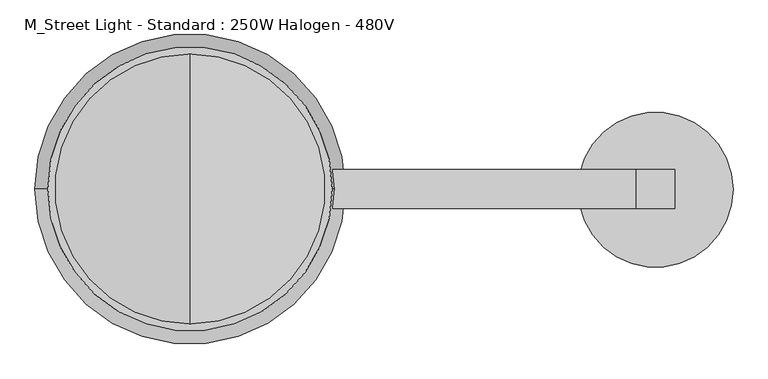
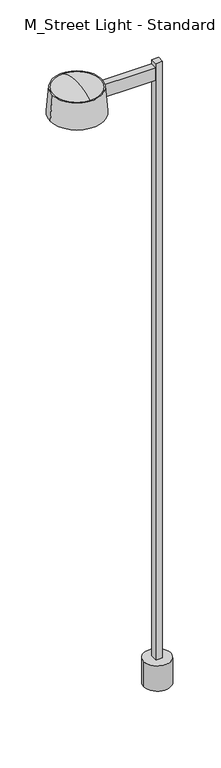
"""IFC4 building model written with IfcOpenShell, lengths in millimetres: light fixture geometry, M_Street Light - Standard : 250W Halogen - 480V."""

from ifc_helpers import new_model, si_unit, point, frame, origin, origin_with_axes, origin_2d, place, context, project, spatial, polyline, circle_curve, ellipse_curve, trimmed, segment, composite_curve, outline, extrude, source, transform, mapped, element, save
from ifc_brep_helpers import plane_surface, revolved_surface, advanced_brep


def m_street_light_standard_250w_halogen_480v_204dbcbb(model_context):
    return source(origin(), model_context, "Body", "SolidModel", [
        extrude(outline(composite_curve([segment(trimmed(circle_curve(origin_2d(), 152.4), [point((-152.4, 0.0))], [point((152.4, 0.0))], False, "CARTESIAN"), True, "CONTINUOUS"), segment(trimmed(circle_curve(origin_2d(), 152.4), [point((152.4, 0.0))], [point((-152.4, 0.0))], False, "CARTESIAN"), True, "CONTINUOUS")], self_intersect=False)), origin_with_axes(), (0.0, 0.0, 1.0), 304.8),
        extrude(outline(polyline([(38.1, 38.1), (38.1, -38.1), (-38.1, -38.1), (-38.1, 38.1), (38.1, 38.1)])), frame((0.0, 0.0, 304.8), z_axis=(0.0, 0.0, 1.0), x_axis=(1.0, 0.0, 0.0)), (0.0, 0.0, 1.0), 7195.2),
        extrude(outline(polyline([(-914.4, 38.1), (-38.1, 38.1), (-38.1, -38.1), (-914.4, -38.1), (-914.4, 38.1)])), frame((0.0, 0.0, 7296.8), z_axis=(0.0, 0.0, 1.0), x_axis=(1.0, 0.0, 0.0)), (0.0, 0.0, 1.0), 152.4),
        advanced_brep(
        [(-1193.8, 0.0, 7500.0), (-635.0, 0.0, 7500.0), (-1219.2, 0.0, 7195.2), (-609.6, 0.0, 7195.2)],
        [
            (0, 1, circle_curve(frame((-914.4, 0.0, 7500.0), z_axis=(0.0, 0.0, 1.0), x_axis=(-1.0, 0.0, 0.0)), 279.4)),
            (1, 0, circle_curve(frame((-914.4, 0.0, 7500.0), z_axis=(0.0, 0.0, 1.0), x_axis=(1.0, 0.0, 0.0)), 279.4)),
            (2, 3, circle_curve(frame((-914.4, 0.0, 7195.2), z_axis=(0.0, 0.0, -1.0), x_axis=(1.0, 0.0, 0.0)), 304.8)),
            (3, 2, circle_curve(frame((-914.4, 0.0, 7195.2), z_axis=(0.0, 0.0, -1.0), x_axis=(-1.0, 0.0, 0.0)), 304.8)),
            (3, 1),
            (0, 2),
        ],
        [
            plane_surface(frame((-914.4, 0.0, 7500.0), z_axis=(0.0, 0.0, 1.0), x_axis=(0.0, -1.0, 0.0))),
            plane_surface(frame((-914.4, 0.0, 7195.2), z_axis=(0.0, 0.0, -1.0), x_axis=(0.0, -1.0, 0.0))),
            revolved_surface(polyline([(-1193.8, 0.0, 7500.0), (-1219.2, 0.0, 7195.2)]), (-914.4, 0.0, 10852.8), (0.0, 0.0, -1.0)),
            revolved_surface(polyline([(-635.0, 0.0, 7500.0), (-609.6, 0.0, 7195.2)]), (-914.4, 0.0, 10852.8), (0.0, 0.0, -1.0)),
        ],
        [
            (0, [[1, 2]]),
            (1, [[3, 4]]),
            (2, [[-4, 5, -1, 6]]),
            (3, [[-3, -6, -2, -5]]),
        ],
    ),
        advanced_brep(
        [(-914.4, -266.7, 7500.0), (-914.4, 266.7, 7500.0), (-914.4, 0.0, 7571.4620496), (-914.4, -228.6332063, 7500.0), (-914.4, 228.6332063, 7500.0), (-914.4, 0.0, 7558.7620496)],
        [
            (0, 1, circle_curve(frame((-914.4, 0.0, 7500.0), z_axis=(0.0, 0.0, 1.0), x_axis=(0.0, 1.0, 0.0)), 266.7)),
            (1, 2, circle_curve(frame((-914.4, -28.9924067, 6929.8609147), z_axis=(1.0, 0.0, 0.0), x_axis=(0.0, 0.0, 1.0)), 642.2558493)),
            (2, 0, circle_curve(frame((-914.4, 28.9924067, 6929.8609147), z_axis=(1.0, 0.0, 0.0), x_axis=(0.0, 0.0, 1.0)), 642.2558493)),
            (1, 0, circle_curve(frame((-914.4, 0.0, 7500.0), z_axis=(0.0, 0.0, 1.0), x_axis=(0.0, 1.0, 0.0)), 266.7)),
            (3, 4, circle_curve(frame((-914.4, 0.0, 7500.0), z_axis=(0.0, 0.0, 1.0), x_axis=(0.0, 1.0, 0.0)), 228.6332063)),
            (4, 1),
            (0, 3),
            (4, 3, circle_curve(frame((-914.4, 0.0, 7500.0), z_axis=(0.0, 0.0, 1.0), x_axis=(0.0, 1.0, 0.0)), 228.6332063)),
            (5, 4),
            (3, 5),
        ],
        [
            revolved_surface(trimmed(ellipse_curve(frame((-914.4, -28.9924067, 6929.8609147), z_axis=(-1.0, 0.0, 0.0), x_axis=(0.0, 0.0, 1.0)), 642.2558493, 642.2558493), [point((-914.4, 0.0, 7571.4620496))], [point((-914.4, 266.7, 7500.0))], True, "CARTESIAN"), (-914.4, 0.0, 7423.8), (0.0, 0.0, -1.0)),
            plane_surface(frame((-914.4, 0.0, 7500.0), z_axis=(0.0, 0.0, -1.0), x_axis=(0.0, 1.0, 0.0))),
            revolved_surface(polyline([(-914.4, 228.6332063, 7500.0), (-914.4, 0.0, 7558.7620496)]), (-914.4, 0.0, 7423.8), (0.0, 0.0, -1.0)),
        ],
        [
            (0, [[1, 2, 3]]),
            (0, [[4, -3, -2]]),
            (1, [[5, 6, -1, 7]]),
            (1, [[8, -7, -4, -6]]),
            (2, [[9, -5, 10]]),
            (2, [[-10, -8, -9]]),
        ],
    ),
        advanced_brep(
        [(-914.4, -228.6332063, 7195.2), (-914.4, 228.6332063, 7195.2), (-914.4, 0.0, 7136.4379504), (-914.4, -266.7, 7195.2), (-914.4, 266.7, 7195.2), (-914.4, 0.0, 7123.7379504)],
        [
            (0, 1, circle_curve(frame((-914.4, 0.0, 7195.2), z_axis=(0.0, 0.0, 1.0), x_axis=(0.0, 1.0, 0.0)), 228.6332063)),
            (1, 2),
            (2, 0),
            (1, 0, circle_curve(frame((-914.4, 0.0, 7195.2), z_axis=(0.0, 0.0, 1.0), x_axis=(0.0, 1.0, 0.0)), 228.6332063)),
            (3, 4, circle_curve(frame((-914.4, 0.0, 7195.2), z_axis=(0.0, 0.0, 1.0), x_axis=(0.0, 1.0, 0.0)), 266.7)),
            (4, 1),
            (0, 3),
            (4, 3, circle_curve(frame((-914.4, 0.0, 7195.2), z_axis=(0.0, 0.0, 1.0), x_axis=(0.0, 1.0, 0.0)), 266.7)),
            (5, 4, circle_curve(frame((-914.4, -28.9924067, 7765.3390853), z_axis=(1.0, 0.0, 0.0), x_axis=(0.0, 0.0, -1.0)), 642.2558493)),
            (3, 5, circle_curve(frame((-914.4, 28.9924067, 7765.3390853), z_axis=(1.0, 0.0, 0.0), x_axis=(0.0, 0.0, -1.0)), 642.2558493)),
        ],
        [
            revolved_surface(polyline([(-914.4, 0.0, 7136.4379504), (-914.4, 228.6332063, 7195.2)]), (-914.4, 0.0, 7271.4), (0.0, 0.0, -1.0)),
            plane_surface(frame((-914.4, 0.0, 7195.2), z_axis=(0.0, 0.0, 1.0), x_axis=(0.0, 1.0, 0.0))),
            revolved_surface(trimmed(ellipse_curve(frame((-914.4, -28.9924067, 7765.3390853), z_axis=(-1.0, 0.0, 0.0), x_axis=(0.0, 0.0, -1.0)), 642.2558493, 642.2558493), [point((-914.4, 266.7, 7195.2))], [point((-914.4, 0.0, 7123.7379504))], True, "CARTESIAN"), (-914.4, 0.0, 7271.4), (0.0, 0.0, -1.0)),
        ],
        [
            (0, [[1, 2, 3]]),
            (0, [[4, -3, -2]]),
            (1, [[5, 6, -1, 7]]),
            (1, [[8, -7, -4, -6]]),
            (2, [[9, -5, 10]]),
            (2, [[-10, -8, -9]]),
        ],
    ),
    ])


if __name__ == "__main__":
    model = new_model("IFC4")
    model_context = context("Model", 3, world=origin())
    ifc_project = project(units=[si_unit("LENGTHUNIT", "METRE", prefix="MILLI")], contexts=[model_context])
    site = spatial("IfcSite", under=ifc_project)
    building = spatial("IfcBuilding", under=site)
    placement = place(None, origin())
    m_street_light_standard_250w_halogen_480v_shape = m_street_light_standard_250w_halogen_480v_204dbcbb(model_context)
    element("IfcLightFixture", 1, ObjectType="M_Street Light - Standard : 250W Halogen - 480V", at=placement, inside=building, context=model_context, shape_type="MappedRepresentation", body=[
        mapped(m_street_light_standard_250w_halogen_480v_shape, transform((0.0, 0.0, 0.0), x_axis=(1.0, 0.0, 0.0), y_axis=(0.0, 1.0, 0.0), z_axis=(0.0, 0.0, 1.0))),
    ])
    save(model, "model.ifc")

# Revit data of these elements
# Type "M_Street Light - Standard : 250W Halogen - 480V"
#   Photometric Web File = "SLS1T4.IES"
#   Lamp = "T-4"
#   Wattage Comments = "250"
#   Wattage = 1000 W
#   built-in parameter 1150110 = 2 (stored number, unit not read)
#   built-in parameter 1114217 = 4 (stored number, unit not read)
#   built-in parameter 1150109 = 2 (stored number, unit not read)
#   built-in parameter 1150113 = 1 (stored number, unit not read)
#   Tilt Angle = -90.00°
#   built-in parameter 1150115 = 1 (stored number, unit not read)
#   built-in parameter 1150105 = 7957.75 (stored number, unit not read)
#   built-in parameter 1150112 = 1 (stored number, unit not read)
#   built-in parameter 1150114 = 1 (stored number, unit not read)
#   built-in parameter 1150107 = 6500 (stored number, unit not read)
#   built-in parameter 1150106 = 79.5775 (stored number, unit not read)
#   Height = 24' - 7.27559"
#   Lumens = 100000 lm
#   built-in parameter 1150104 = 9.2903 (stored number, unit not read)
#   Voltage = 480 V
#   built-in parameter 1114218 = 1 (stored number, unit not read)
#   built-in parameter 1150133 = 10 (stored number, unit not read)
#   Apparent Load = 250 VA
#   built-in parameter 1150134 = 1
#   built-in parameter 1150137 = 1
#   Color Filter = 16777215
#   Number of poles = 3
#   Stand Material = Steel, Paint Finish, Dark Gray, Matte
#   Shade Material = Steel, Paint Finish, Dark Gray, Matte
#   Load Classification = Lighting - Exterior
#   Diffuser Material = Glass, Frosted
#   Dimming Lamp Color Temperature Shift = (empty or 0)
#   Default Elevation = 0
# Element 1 (IfcLightFixture, "M_Street Light - Standard : 250W Halogen - 480V")
#   Materials on its faces: "Steel, Paint Finish, Dark Gray, Matte", "Glass, Frosted"
# Materials
#   "Steel, Paint Finish, Dark Gray, Matte": class "Metal", colour RGB 98 98 98, transparency 0, Description = "Steel, paint finish, dark gray, matte", Cost = 0
#   "Glass, Frosted": class "Glass", colour RGB 249 250 249, transparency 0.8, Description = "physical material", Cost = 0
